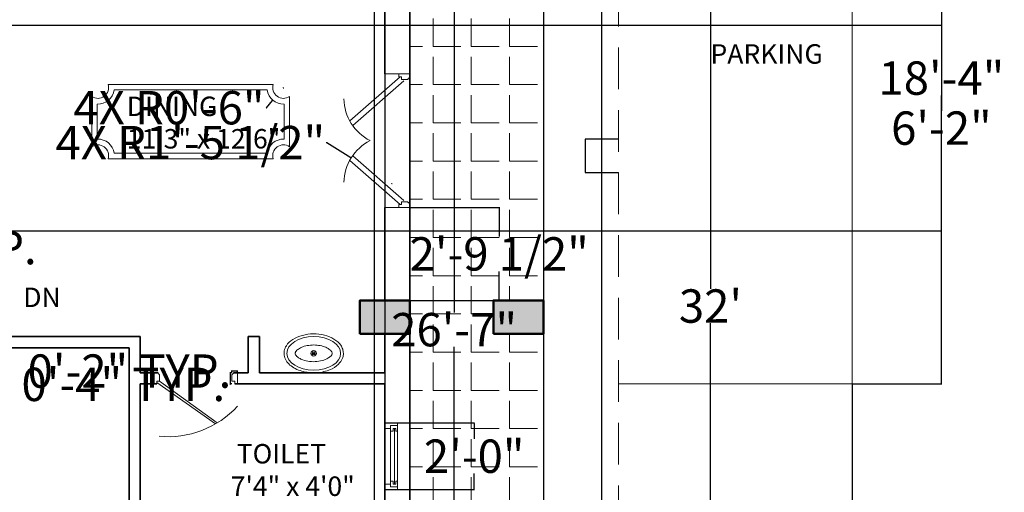
# Model space of a CAD drawing. Units: inches. Extents: x 1063 to 2718, y 423 to 1923.
# Tile 3 of 7: x 1268 to 1622, y 692 to 862. Entities that reach past the tile are written whole.
import ezdxf

# ---------------------------------------------------------------- set-up
doc = ezdxf.new("R2010")
doc.units = ezdxf.units.IN
doc.header["$LTSCALE"] = 6
doc.header["$MEASUREMENT"] = 0
doc.linetypes.add('HIDDEN', pattern=[0.375, 0.25, -0.125])
for name, color, linetype, lineweight in [('A-ANNO-DIMS', 2, 'Continuous', 18), ('A-ANNO-TEXT', 7, 'Continuous', 18), ('A-AREA-IDEN', 7, 'Continuous', 18), ('A-COLS', 7, 'Continuous', 50), ('A-COLS-PATT', 252, 'Continuous', 13), ('A-DOOR', 2, 'Continuous', 18), ('A-FLOR', 7, 'Continuous', 25), ('A-FLOR-FIXT', 4, 'Continuous', 18), ('A-FLOR-PATT', 9, 'Continuous', 13), ('A-FURN', 4, 'Continuous', 18), ('A-GLAZ', 4, 'Continuous', 18), ('A-WALL', 7, 'Continuous', 35), ('C-PKNG', 7, 'Continuous', 18), ('C-PROP', 7, 'Continuous', 25), ('C-PROP-HIDN', 7, 'HIDDEN', 18)]:
    doc.layers.add(name, color=color, linetype=linetype, lineweight=lineweight)
doc.styles.get("Standard").update_dxf_attribs({"font": 'arial.ttf'})
doc.dimstyles.get("Standard").update_dxf_attribs({"dimtxt": 12, "dimasz": 0.18, "dimexe": 0.18, "dimexo": 0.0625, "dimgap": 0.09, "dimtad": 0, "dimtih": 1, "dimtoh": 1, "dimdec": 1, "dimzin": 0, "dimdsep": 46, "dimlunit": 3, "dimtxsty": 'Standard', "dimcen": 0.09, "dimadec": 0, "dimazin": 0, "dimtfac": 1, "dimtdec": 1, "dimtofl": 0, "dimtmove": 0, "dimatfit": 3, "dimfxl": 1, "dimtolj": 1, "dimtzin": 0, "dimarcsym": 0})

# ---------------------------------------------------------------- blocks, each defined once
blk = doc.blocks.new('*D3')
at = {"layer": 'A-ANNO-DIMS', "color": 0, "lineweight": -2, "ltscale": 6, "transparency": 16777216}
for p, q in [((1482.99, 951.12), (1516.18, 951.12)), ((1516, 950.94), (1516, 765.34)), ((1516, 567.3), (1516, 752.9)), ((1482.99, 567.12), (1516.18, 567.12))]:
    blk.add_line(p, q, dxfattribs=at)
at = {"layer": 'A-ANNO-DIMS', "color": 0, "ltscale": 6, "transparency": 16777216}
for points in [[(1515.97, 950.94), (1516.03, 950.94), (1516, 951.12)], [(1515.97, 567.3), (1516.03, 567.3), (1516, 567.12)]]:
    blk.add_solid(points, dxfattribs=at)
at = {"layer": 'Defpoints', "color": 0, "ltscale": 6, "transparency": 16777216}
for p in [(1482.93, 951.12), (1516, 951.12), (1482.93, 567.12)]:
    blk.add_point(p, dxfattribs=at)
at = {"layer": 'A-ANNO-DIMS', "color": 0, "ltscale": 6, "transparency": 16777216, "insert": (1516, 759.12), "char_height": 12, "attachment_point": 5}
blk.add_mtext("\\A1;32'", dxfattribs=at)
blk = doc.blocks.new('DOOR-48-DOUBLE-SWING')
at = {"ltscale": 6}
for p, q in [((20.22, 47), (2.07, 31.16)), ((19.72, 48), (19.72, 47)), ((19.72, 47), (20.72, 47)), ((20.72, 47), (20.72, 46)), ((23.19, 46.24), (23.03, 46.24)), ((23.03, 46.24), (23.03, 46)), ((23.72, 46.54), (23.39, 46.54)), ((23.39, 46.54), (23.39, 46.44)), ((21.53, 45.49), (3.14, 29.43)), ((20.72, 46), (23.03, 46)), ((21.53, 2.51), (3.14, 18.57)), ((20.22, 1), (2.07, 16.84)), ((19.72, 0), (19.72, 1)), ((19.72, 1), (20.72, 1)), ((20.72, 1), (20.72, 2)), ((20.72, 2), (23.03, 2)), ((23.03, 1.76), (23.03, 2)), ((23.19, 1.76), (23.03, 1.76)), ((23.39, 1.46), (23.39, 1.56)), ((23.72, 1.46), (23.39, 1.46))]:
    blk.add_line(p, q, dxfattribs=at)
for p, q in [((14.72, 48), (23.72, 48)), ((23.72, 0), (14.72, 0))]:
    blk.add_line(p, q)
for centre, radius, start, end in [((23.19, 46.44), 0.2, 270, 0), ((17.26, 39.37), 17.27, 181.2158, 242.8966), ((17.26, 8.63), 17.27, 117.1034, 178.7842), ((23.19, 1.56), 0.2, 0, 90)]:
    blk.add_arc(centre, radius, start, end, dxfattribs=at)
blk = doc.blocks.new('DOOR-JAMB-4')
at = {"ltscale": 6}
for p, q in [((0, 0), (0, 4)), ((1, 4), (1, 3)), ((1, 3), (2, 3)), ((1.46, 0), (1.46, 0.33)), ((1.46, 0.33), (1.56, 0.33)), ((1.76, 0.53), (1.76, 0.69)), ((1.76, 0.69), (2, 0.69)), ((2, 3), (2, 0.69))]:
    blk.add_line(p, q, dxfattribs=at)
blk.add_arc((1.56, 0.53), 0.2, 270, 0, dxfattribs=at)
blk = doc.blocks.new('COLUMN-18X12')
blk.add_lwpolyline([(0, 0), (18, 0), (18, 12), (0, 12)], close=True)
blk = doc.blocks.new('PIER-12X12-INLINE')
blk.add_lwpolyline([(0, 0), (12, 0), (12, 12), (0, 12)])
blk = doc.blocks.new('*D28')
at = {"layer": 'A-ANNO-DIMS', "color": 0, "lineweight": -2, "ltscale": 6, "transparency": 16777216}
for p, q in [((1174.86, 804.12), (1167.55, 804.12)), ((1167.73, 803.94), (1167.73, 786.42)), ((1167.73, 756.3), (1167.73, 773.82)), ((1174.86, 756.12), (1167.55, 756.12))]:
    blk.add_line(p, q, dxfattribs=at)
at = {"layer": 'A-ANNO-DIMS', "color": 0, "ltscale": 6, "transparency": 16777216}
for points in [[(1167.7, 803.94), (1167.76, 803.94), (1167.73, 804.12)], [(1167.7, 756.3), (1167.76, 756.3), (1167.73, 756.12)]]:
    blk.add_solid(points, dxfattribs=at)
at = {"layer": 'Defpoints', "color": 0, "ltscale": 6, "transparency": 16777216}
for p in [(1174.93, 804.12), (1167.73, 756.12), (1174.93, 756.12)]:
    blk.add_point(p, dxfattribs=at)
at = {"layer": 'A-ANNO-DIMS', "color": 0, "ltscale": 6, "transparency": 16777216, "insert": (1167.73, 780.12), "char_height": 12, "attachment_point": 5}
blk.add_mtext('\\A1;SLIDING WINDOW 4\'-0" TYP.', dxfattribs=at)
blk = doc.blocks.new('*D32')
at = {"layer": 'A-ANNO-DIMS', "color": 0, "lineweight": -2, "ltscale": 6, "transparency": 16777216}
for p, q in [((1343.86, 735.12), (1343.15, 735.12)), ((1343.33, 734.94), (1343.33, 731.3)), ((1343.86, 731.12), (1343.15, 731.12)), ((1343.33, 730.94), (1343.15, 730.94)), ((1343.33, 731.12), (1343.33, 730.94))]:
    blk.add_line(p, q, dxfattribs=at)
at = {"layer": 'A-ANNO-DIMS', "color": 0, "ltscale": 6, "transparency": 16777216}
for points in [[(1343.3, 734.94), (1343.36, 734.94), (1343.33, 735.12)], [(1343.3, 731.3), (1343.36, 731.3), (1343.33, 731.12)]]:
    blk.add_solid(points, dxfattribs=at)
at = {"layer": 'Defpoints', "color": 0, "ltscale": 6, "transparency": 16777216}
for p in [(1343.93, 735.12), (1343.33, 731.12), (1343.93, 731.12)]:
    blk.add_point(p, dxfattribs=at)
at = {"layer": 'A-ANNO-DIMS', "color": 0, "ltscale": 6, "transparency": 16777216, "insert": (1281.68, 730.94), "char_height": 12, "attachment_point": 5}
blk.add_mtext('\\A1;JAMB 0\'-4" TYP.', dxfattribs=at)
blk = doc.blocks.new('*D33')
at = {"layer": 'A-ANNO-DIMS', "color": 0, "lineweight": -2, "ltscale": 6, "transparency": 16777216}
for p, q in [((1343.93, 735.72), (1343.75, 735.72)), ((1343.93, 735.18), (1343.93, 735.9)), ((1345.75, 735.72), (1344.11, 735.72)), ((1345.93, 735.18), (1345.93, 735.9))]:
    blk.add_line(p, q, dxfattribs=at)
at = {"layer": 'A-ANNO-DIMS', "color": 0, "ltscale": 6, "transparency": 16777216}
for points in [[(1344.11, 735.75), (1344.11, 735.69), (1343.93, 735.72)], [(1345.75, 735.75), (1345.75, 735.69), (1345.93, 735.72)]]:
    blk.add_solid(points, dxfattribs=at)
at = {"layer": 'Defpoints', "color": 0, "ltscale": 6, "transparency": 16777216}
for p in [(1343.93, 735.72), (1343.93, 735.12), (1345.93, 735.12)]:
    blk.add_point(p, dxfattribs=at)
at = {"layer": 'A-ANNO-DIMS', "color": 0, "ltscale": 6, "transparency": 16777216, "insert": (1307.08, 735.72), "char_height": 12, "attachment_point": 5}
blk.add_mtext('\\A1;0\'-2" TYP.', dxfattribs=at)
blk = doc.blocks.new('*D42')
at = {"layer": 'A-ANNO-DIMS', "color": 0, "lineweight": -2, "ltscale": 6, "transparency": 16777216}
for p, q in [((1265.93, 901.06), (1265.93, 895.69)), ((1300.93, 901.06), (1300.93, 895.69)), ((1266.11, 895.87), (1300.75, 895.87)), ((1300.93, 895.87), (1301.11, 895.87))]:
    blk.add_line(p, q, dxfattribs=at)
at = {"layer": 'A-ANNO-DIMS', "color": 0, "ltscale": 6, "transparency": 16777216}
for points in [[(1266.11, 895.9), (1266.11, 895.84), (1265.93, 895.87)], [(1300.75, 895.9), (1300.75, 895.84), (1300.93, 895.87)]]:
    blk.add_solid(points, dxfattribs=at)
at = {"layer": 'Defpoints', "color": 0, "ltscale": 6, "transparency": 16777216}
for p in [(1265.93, 901.12), (1300.93, 901.12), (1300.93, 895.87)]:
    blk.add_point(p, dxfattribs=at)
at = {"layer": 'A-ANNO-DIMS', "color": 0, "ltscale": 6, "transparency": 16777216, "insert": (1398.77, 895.87), "char_height": 12, "attachment_point": 5}
blk.add_mtext('\\A1;SINGLE LEAF 2\'-11" TYP.', dxfattribs=at)
blk = doc.blocks.new('*D49')
at = {"layer": 'A-ANNO-DIMS', "color": 0, "lineweight": -2, "ltscale": 6, "transparency": 16777216}
for p, q in [((1566.99, 951.12), (1599.21, 951.12)), ((1599.03, 950.94), (1599.03, 847.34)), ((1599.03, 731.3), (1599.03, 834.9)), ((1566.99, 731.12), (1599.21, 731.12))]:
    blk.add_line(p, q, dxfattribs=at)
at = {"layer": 'A-ANNO-DIMS', "color": 0, "ltscale": 6, "transparency": 16777216}
for points in [[(1599, 950.94), (1599.06, 950.94), (1599.03, 951.12)], [(1599, 731.3), (1599.06, 731.3), (1599.03, 731.12)]]:
    blk.add_solid(points, dxfattribs=at)
at = {"layer": 'Defpoints', "color": 0, "ltscale": 6, "transparency": 16777216}
for p in [(1566.93, 951.12), (1599.03, 951.12), (1566.93, 731.12)]:
    blk.add_point(p, dxfattribs=at)
at = {"layer": 'A-ANNO-DIMS', "color": 0, "ltscale": 6, "transparency": 16777216, "insert": (1599.03, 841.12), "char_height": 12, "attachment_point": 5}
blk.add_mtext('\\A1;18\'-4"', dxfattribs=at)
blk = doc.blocks.new('*D50')
at = {"layer": 'A-ANNO-DIMS', "color": 0, "lineweight": -2, "ltscale": 6, "transparency": 16777216}
for p, q in [((1566.93, 731.06), (1566.93, 431.18)), ((1150.93, 567.06), (1150.93, 431.18)), ((1151.11, 431.36), (1338.23, 431.36)), ((1566.75, 431.36), (1379.62, 431.36))]:
    blk.add_line(p, q, dxfattribs=at)
at = {"layer": 'A-ANNO-DIMS', "color": 0, "ltscale": 6, "transparency": 16777216}
for points in [[(1151.11, 431.39), (1151.11, 431.33), (1150.93, 431.36)], [(1566.75, 431.39), (1566.75, 431.33), (1566.93, 431.36)]]:
    blk.add_solid(points, dxfattribs=at)
at = {"layer": 'Defpoints', "color": 0, "ltscale": 6, "transparency": 16777216}
for p in [(1566.93, 731.12), (1150.93, 567.12), (1566.93, 431.36)]:
    blk.add_point(p, dxfattribs=at)
at = {"layer": 'A-ANNO-DIMS', "color": 0, "ltscale": 6, "transparency": 16777216, "insert": (1358.93, 431.36), "char_height": 12, "attachment_point": 5}
blk.add_mtext('\\A1;34\'-8"', dxfattribs=at)
blk = doc.blocks.new('*D52')
at = {"layer": 'A-ANNO-DIMS', "color": 0, "lineweight": -2, "ltscale": 6, "transparency": 16777216}
for p, q in [((1455.86, 910.12), (1423.65, 910.12)), ((1423.83, 909.94), (1423.83, 756.84)), ((1423.83, 591.3), (1423.83, 744.4)), ((1455.86, 591.12), (1423.65, 591.12))]:
    blk.add_line(p, q, dxfattribs=at)
at = {"layer": 'A-ANNO-DIMS', "color": 0, "ltscale": 6, "transparency": 16777216}
for points in [[(1423.8, 909.94), (1423.86, 909.94), (1423.83, 910.12)], [(1423.8, 591.3), (1423.86, 591.3), (1423.83, 591.12)]]:
    blk.add_solid(points, dxfattribs=at)
at = {"layer": 'Defpoints', "color": 0, "ltscale": 6, "transparency": 16777216}
for p in [(1423.83, 910.12), (1455.93, 910.12), (1455.93, 591.12)]:
    blk.add_point(p, dxfattribs=at)
at = {"layer": 'A-ANNO-DIMS', "color": 0, "ltscale": 6, "transparency": 16777216, "insert": (1423.83, 750.62), "char_height": 12, "attachment_point": 5}
blk.add_mtext('\\A1;26\'-7"', dxfattribs=at)
blk = doc.blocks.new('*D54')
at = {"layer": 'A-ANNO-DIMS', "color": 0, "lineweight": -2, "ltscale": 6, "transparency": 16777216}
for p, q in [((1227.99, 860.12), (1599.21, 860.12)), ((1599.03, 859.94), (1599.03, 829.34)), ((1599.03, 786.3), (1599.03, 816.9)), ((1227.99, 786.12), (1599.21, 786.12))]:
    blk.add_line(p, q, dxfattribs=at)
at = {"layer": 'A-ANNO-DIMS', "color": 0, "ltscale": 6, "transparency": 16777216}
for points in [[(1599, 859.94), (1599.06, 859.94), (1599.03, 860.12)], [(1599, 786.3), (1599.06, 786.3), (1599.03, 786.12)]]:
    blk.add_solid(points, dxfattribs=at)
at = {"layer": 'Defpoints', "color": 0, "ltscale": 6, "transparency": 16777216}
for p in [(1227.93, 860.12), (1227.93, 786.12), (1599.03, 786.12)]:
    blk.add_point(p, dxfattribs=at)
at = {"layer": 'A-ANNO-DIMS', "color": 0, "ltscale": 6, "transparency": 16777216, "insert": (1599.03, 823.12), "char_height": 12, "attachment_point": 5}
blk.add_mtext('\\A1;6\'-2"', dxfattribs=at)
blk = doc.blocks.new('*D65')
at = {"layer": 'A-ANNO-DIMS', "color": 0, "lineweight": -2, "ltscale": 6, "transparency": 16777216}
for p, q in [((1395.08, 961.04), (1395.08, 431.18)), ((1398.93, 954.06), (1398.93, 431.18)), ((1395.26, 431.36), (1398.75, 431.36)), ((1398.93, 431.36), (1399.11, 431.36))]:
    blk.add_line(p, q, dxfattribs=at)
at = {"layer": 'A-ANNO-DIMS', "color": 0, "ltscale": 6, "transparency": 16777216}
for points in [[(1395.26, 431.39), (1395.26, 431.33), (1395.08, 431.36)], [(1398.75, 431.39), (1398.75, 431.33), (1398.93, 431.36)]]:
    blk.add_solid(points, dxfattribs=at)
at = {"layer": 'Defpoints', "color": 0, "ltscale": 6, "transparency": 16777216}
for p in [(1395.08, 961.11), (1398.93, 954.12), (1398.93, 431.36)]:
    blk.add_point(p, dxfattribs=at)
at = {"layer": 'A-ANNO-DIMS', "color": 0, "ltscale": 6, "transparency": 16777216, "insert": (1415.15, 431.36), "char_height": 12, "attachment_point": 5}
blk.add_mtext('\\A1;0\'-4"', dxfattribs=at)
blk = doc.blocks.new('*D70')
at = {"layer": 'A-ANNO-DIMS', "color": 0, "lineweight": -2, "ltscale": 6, "transparency": 16777216}
for p, q in [((1398.99, 717.1), (1431.21, 717.1)), ((1431.03, 716.92), (1431.03, 711.32)), ((1431.03, 693.28), (1431.03, 698.88)), ((1398.99, 693.1), (1431.21, 693.1))]:
    blk.add_line(p, q, dxfattribs=at)
at = {"layer": 'A-ANNO-DIMS', "color": 0, "ltscale": 6, "transparency": 16777216}
for points in [[(1431, 716.92), (1431.06, 716.92), (1431.03, 717.1)], [(1431, 693.28), (1431.06, 693.28), (1431.03, 693.1)]]:
    blk.add_solid(points, dxfattribs=at)
at = {"layer": 'Defpoints', "color": 0, "ltscale": 6, "transparency": 16777216}
for p in [(1398.93, 717.1), (1398.93, 693.1), (1431.03, 693.1)]:
    blk.add_point(p, dxfattribs=at)
at = {"layer": 'A-ANNO-DIMS', "color": 0, "ltscale": 6, "transparency": 16777216, "insert": (1431.03, 705.1), "char_height": 12, "attachment_point": 5}
blk.add_mtext('\\A1;2\'-0"', dxfattribs=at)
blk = doc.blocks.new('*D71')
at = {"layer": 'A-ANNO-DIMS', "color": 0, "lineweight": -2, "ltscale": 6, "transparency": 16777216}
for p, q in [((1407.99, 794.62), (1440.21, 794.62)), ((1440.03, 794.44), (1440.03, 784.16)), ((1440.03, 761.29), (1440.03, 771.57)), ((1407.99, 761.11), (1440.21, 761.11))]:
    blk.add_line(p, q, dxfattribs=at)
at = {"layer": 'A-ANNO-DIMS', "color": 0, "ltscale": 6, "transparency": 16777216}
for points in [[(1440, 794.44), (1440.06, 794.44), (1440.03, 794.62)], [(1440, 761.29), (1440.06, 761.29), (1440.03, 761.11)]]:
    blk.add_solid(points, dxfattribs=at)
at = {"layer": 'Defpoints', "color": 0, "ltscale": 6, "transparency": 16777216}
for p in [(1407.93, 794.62), (1407.93, 761.11), (1440.03, 761.11)]:
    blk.add_point(p, dxfattribs=at)
at = {"layer": 'A-ANNO-DIMS', "color": 0, "ltscale": 6, "transparency": 16777216, "insert": (1440.03, 777.87), "char_height": 12, "attachment_point": 5}
blk.add_mtext('\\A1;2\'-9 1/2"', dxfattribs=at)
blk = doc.blocks.new('*D74')
at = {"layer": 'A-ANNO-DIMS', "color": 0, "lineweight": -2, "ltscale": 6, "transparency": 16777216}
for p, q in [((1377.88, 817.91), (1378.06, 817.91)), ((1378.06, 817.91), (1386.68, 812.51)), ((1401.38, 803.25), (1401.56, 803.25)), ((1401.47, 803.16), (1401.47, 803.34))]:
    blk.add_line(p, q, dxfattribs=at)
at = {"layer": 'A-ANNO-DIMS', "color": 0, "ltscale": 6, "transparency": 16777216}
blk.add_solid([(1386.7, 812.53), (1386.67, 812.48), (1386.84, 812.41)], dxfattribs=at)
at = {"layer": 'Defpoints', "color": 0, "ltscale": 6, "transparency": 16777216}
for p in [(1386.84, 812.41), (1401.47, 803.25)]:
    blk.add_point(p, dxfattribs=at)
at = {"layer": 'A-ANNO-DIMS', "color": 0, "ltscale": 6, "transparency": 16777216, "insert": (1328.98, 817.91), "char_height": 12, "attachment_point": 5}
blk.add_mtext('\\A1;4X R1\'-5 1/2"', dxfattribs=at)
blk = doc.blocks.new('*D75')
at = {"layer": 'A-ANNO-DIMS', "color": 0, "lineweight": -2, "ltscale": 6, "transparency": 16777216}
for p, q in [((1362.37, 837.65), (1362.55, 837.65)), ((1362.46, 837.56), (1362.46, 837.74)), ((1356.4, 830.45), (1358.56, 833.01)), ((1356.22, 830.45), (1356.4, 830.45))]:
    blk.add_line(p, q, dxfattribs=at)
at = {"layer": 'A-ANNO-DIMS', "color": 0, "ltscale": 6, "transparency": 16777216}
blk.add_solid([(1358.54, 833.03), (1358.58, 832.99), (1358.67, 833.15)], dxfattribs=at)
at = {"layer": 'Defpoints', "color": 0, "ltscale": 6, "transparency": 16777216}
for p in [(1362.46, 837.65), (1358.67, 833.15)]:
    blk.add_point(p, dxfattribs=at)
at = {"layer": 'A-ANNO-DIMS', "color": 0, "ltscale": 6, "transparency": 16777216, "insert": (1321.3, 830.45), "char_height": 12, "attachment_point": 5}
blk.add_mtext('\\A1;4X R0\'-6"', dxfattribs=at)

msp = doc.modelspace()

# ---------------------------------------------------------------- hatches: boundary and pattern name
at = {"layer": 'A-COLS-PATT', "ltscale": 6}
h = msp.add_hatch(color=256, dxfattribs=at)
h.dxf.hatch_style = 1
h.paths.add_polyline_path([(1192.93, 603.12), (1174.93, 603.12), (1174.93, 591.12), (1192.93, 591.12)])
h.paths.add_polyline_path([(1407.93, 603.12), (1389.93, 603.12), (1389.93, 591.12), (1407.93, 591.12)])
h.paths.add_polyline_path([(1192.93, 756.12), (1174.93, 756.12), (1174.93, 744.12), (1192.93, 744.12)])
h.paths.add_polyline_path([(1407.93, 761.11), (1389.93, 761.11), (1389.93, 749.11), (1407.93, 749.11)])
h.paths.add_polyline_path([(1455.93, 761.11), (1437.93, 761.11), (1437.93, 749.11), (1455.93, 749.11)])
h.paths.add_polyline_path([(1455.93, 910.12), (1437.93, 910.12), (1437.93, 898.12), (1455.93, 898.12)])
h.paths.add_polyline_path([(1407.93, 910.12), (1389.93, 910.12), (1389.93, 898.12), (1407.93, 898.12)])
h.paths.add_polyline_path([(1192.93, 910.12), (1174.93, 910.12), (1174.93, 898.12), (1192.93, 898.12)])
h.paths.add_polyline_path([(1192.93, 1055.12), (1174.93, 1055.12), (1174.93, 1043.12), (1192.93, 1043.12)])
h.paths.add_polyline_path([(1407.93, 1055.12), (1389.93, 1055.12), (1389.93, 1043.12), (1407.93, 1043.12)])
at = {"layer": 'A-FLOR-PATT', "ltscale": 6}
h = msp.add_hatch(dxfattribs=at)
h.set_pattern_fill('ANGLE', color=256, scale=50)
h.set_pattern_definition([(0, (0, 0), (0, 13.75), [10, -3.75]), (90, (0, 0), (-13.75, 8e-16), [10, -3.75])])
h.paths.add_polyline_path([(1455.93, 749.11), (1437.93, 749.11), (1437.93, 761.11), (1455.93, 761.11), (1455.93, 868.12), (1407.93, 868.12), (1407.93, 595.12), (1455.93, 595.12)])
h.paths.add_polyline_path([(1377.93, 674.12), (1315.93, 674.12), (1315.93, 600.12), (1377.93, 600.12)])

# ---------------------------------------------------------------- linework, layer by layer
at = {"layer": 'A-DOOR', "ltscale": 6}
for p, q in [((1316.93, 731.62), (1338.02, 716.72)), ((1317.93, 732.12), (1338.68, 717.11))]:
    msp.add_line(p, q, dxfattribs=at)
msp.add_arc((1320.91, 746.15), 34.04, 264.6951, 317.3946, dxfattribs=at)
at = {"layer": 'A-FLOR'}
msp.add_line((1455.93, 898.12), (1455.93, 591.12), dxfattribs=at)
at = {"layer": 'A-FLOR-FIXT', "ltscale": 6}
for p, q in [((1373.88, 742.1), (1372.8, 742.1)), ((1373.34, 742.64), (1373.34, 741.56))]:
    msp.add_line(p, q, dxfattribs=at)
for radius in [0.987, 0.539]:
    msp.add_circle((1373.34, 742.1), radius, dxfattribs=at)
msp.add_ellipse((1373.34, 742.1), major_axis=(9.67, 0), ratio=0.620608, dxfattribs=at)
for points, knots in [([(1384.01, 742.1), (1384.01, 742.61), (1383.92, 743.12), (1383.61, 744.09), (1383.37, 744.56), (1382.48, 745.87), (1381.64, 746.62), (1379.63, 747.85), (1378.45, 748.32), (1375.92, 748.96), (1374.56, 749.11), (1371.86, 749.09), (1370.51, 748.91), (1368, 748.24), (1366.84, 747.75), (1364.87, 746.49), (1364.06, 745.72), (1363.13, 744.25), (1362.87, 743.61), (1362.63, 742.29), (1362.65, 741.61), (1362.97, 740.3), (1363.27, 739.68), (1364.09, 738.53), (1364.6, 738.01), (1366.41, 736.62), (1367.96, 735.93), (1371.37, 735.12), (1373.22, 735), (1376.8, 735.37), (1378.51, 735.85), (1381.08, 737.16), (1382.04, 737.9), (1383.22, 739.35), (1383.57, 739.99), (1383.93, 741.13), (1384.01, 741.61), (1384.01, 742.1)], [0, 0, 0, 0, 0.199891, 0.199891, 0.399781, 0.399781, 0.794265, 0.794265, 1.188748, 1.188748, 1.583232, 1.583232, 1.977715, 1.977715, 2.372199, 2.372199, 2.766682, 2.766682, 3.030116, 3.030116, 3.293549, 3.293549, 3.556982, 3.556982, 3.820416, 3.820416, 4.347819, 4.347819, 4.875222, 4.875222, 5.402625, 5.402625, 5.816568, 5.816568, 6.091003, 6.091003, 6.283185, 6.283185, 6.283185, 6.283185]), ([(1380.01, 742.1), (1380.01, 742.17), (1380, 742.25), (1379.94, 742.43), (1379.9, 742.54), (1379.73, 742.81), (1379.61, 742.96), (1379.28, 743.3), (1379.08, 743.47), (1378.4, 743.94), (1377.86, 744.22), (1376.59, 744.68), (1375.87, 744.87), (1374.35, 745.09), (1373.55, 745.13), (1371.97, 745.05), (1371.2, 744.94), (1369.77, 744.59), (1369.13, 744.35), (1368.05, 743.81), (1367.63, 743.51), (1367.1, 743.01), (1366.95, 742.81), (1366.75, 742.48), (1366.71, 742.35), (1366.67, 742.15), (1366.67, 742.07), (1366.7, 741.87), (1366.74, 741.75), (1366.92, 741.43), (1367.07, 741.23), (1367.51, 740.81), (1367.8, 740.58), (1368.52, 740.15), (1368.94, 739.94), (1370.14, 739.5), (1370.97, 739.3), (1372.71, 739.09), (1373.63, 739.07), (1375.39, 739.24), (1376.24, 739.42), (1377.73, 739.92), (1378.36, 740.24), (1379.18, 740.8), (1379.44, 741.04), (1379.79, 741.47), (1379.89, 741.65), (1379.99, 741.92), (1380.01, 742.01), (1380.01, 742.1)], [0, 0, 0, 0, 0.18324, 0.18324, 0.366481, 0.366481, 0.549721, 0.549721, 0.732962, 0.732962, 1.037063, 1.037063, 1.341164, 1.341164, 1.645265, 1.645265, 1.949367, 1.949367, 2.253468, 2.253468, 2.557569, 2.557569, 2.788449, 2.788449, 3.019329, 3.019329, 3.250209, 3.250209, 3.481089, 3.481089, 3.711969, 3.711969, 3.942849, 3.942849, 4.173729, 4.173729, 4.518554, 4.518554, 4.863378, 4.863378, 5.208203, 5.208203, 5.553027, 5.553027, 5.802313, 5.802313, 6.051598, 6.051598, 6.283185, 6.283185, 6.283185, 6.283185])]:
    msp.add_open_spline(points, degree=3, knots=knots, dxfattribs=at)
at = {"layer": 'A-FURN', "ltscale": 6}
for p, q in [((1299.39, 838.86), (1358.82, 838.86)), ((1301.58, 836.86), (1356.63, 836.86)), ((1293.53, 816.41), (1293.53, 834.52)), ((1364.68, 834.52), (1364.68, 816.41)), ((1295.53, 819.15), (1295.53, 831.77)), ((1362.68, 831.77), (1362.68, 819.15)), ((1358.82, 812.06), (1299.39, 812.06)), ((1356.63, 814.06), (1301.58, 814.06))]:
    msp.add_line(p, q, dxfattribs=at)
for centre, radius, start, end in [((1295.74, 837.65), 3.84, 234.8003, 18.3164), ((1295.74, 837.65), 5.89, 267.9212, 352.2551), ((1362.46, 837.65), 5.89, 187.7449, 272.0788), ((1362.46, 837.65), 3.84, 161.6836, 305.1997), ((1295.74, 813.27), 5.89, 7.7449, 92.0788), ((1362.46, 813.27), 5.89, 87.9212, 172.2551), ((1295.74, 813.27), 3.84, 341.6836, 125.1997), ((1362.46, 813.27), 3.84, 54.8003, 198.3164)]:
    msp.add_arc(centre, radius, start, end, dxfattribs=at)
at = {"layer": 'A-GLAZ', "ltscale": 6}
for p, q in [((1398.93, 717.1), (1398.93, 715.1)), ((1400.93, 715.1), (1400.93, 716.1)), ((1400.93, 716.1), (1403.43, 716.1)), ((1403.43, 717.1), (1403.43, 693.1)), ((1403.43, 694.1), (1403.43, 716.1)), ((1398.93, 715.1), (1400.93, 715.1)), ((1400.93, 695.1), (1400.93, 715.1)), ((1400.93, 715.1), (1400.93, 714.1)), ((1400.93, 714.1), (1401.93, 714.1)), ((1401.93, 714.1), (1401.93, 715.1)), ((1401.93, 715.1), (1402.93, 715.1)), ((1402.43, 695.1), (1402.43, 715.1)), ((1402.93, 715.1), (1402.93, 714.1)), ((1402.93, 714.1), (1403.43, 714.1)), ((1398.93, 693.1), (1398.93, 695.1)), ((1398.93, 695.1), (1400.93, 695.1)), ((1400.93, 695.1), (1400.93, 696.1)), ((1400.93, 696.1), (1401.93, 696.1)), ((1400.93, 695.1), (1400.93, 694.1)), ((1400.93, 694.1), (1403.43, 694.1)), ((1401.93, 696.1), (1401.93, 695.1)), ((1401.93, 695.1), (1402.93, 695.1)), ((1402.93, 695.1), (1402.93, 696.1)), ((1402.93, 696.1), (1403.43, 696.1))]:
    msp.add_line(p, q, dxfattribs=at)
msp.add_lwpolyline([(1407.93, 693.1), (1407.93, 717.1), (1398.93, 717.1), (1398.93, 693.1)], close=True, dxfattribs=at)
at = {"layer": 'A-WALL', "ltscale": 6}
for p, q in [((1407.93, 1055.12), (1407.93, 591.12)), ((1349.83, 735.12), (1349.83, 748.12)), ((1349.83, 748.12), (1353.83, 748.12)), ((1353.83, 735.12), (1353.83, 748.12)), ((1398.93, 731.12), (1344.93, 731.12))]:
    msp.add_line(p, q, dxfattribs=at)
at = {"layer": 'A-WALL'}
for p, q in [((1398.93, 898.12), (1398.93, 842.62)), ((1398.93, 794.62), (1398.93, 761.11)), ((1310.93, 748.12), (1192.93, 748.12)), ((1310.93, 748.12), (1310.93, 735.12)), ((1398.93, 749.11), (1398.93, 735.12)), ((1306.93, 744.12), (1183.93, 744.12)), ((1306.93, 744.12), (1306.93, 655.12)), ((1310.93, 735.12), (1317.39, 735.12)), ((1344.46, 735.12), (1349.83, 735.12)), ((1353.83, 735.12), (1398.93, 735.12)), ((1310.93, 731.12), (1316.93, 731.12)), ((1310.93, 731.12), (1310.93, 683.12)), ((1398.93, 731.12), (1398.93, 683.12))]:
    msp.add_line(p, q, dxfattribs=at)
at = {"layer": 'C-PKNG', "ltscale": 6}
for p, q in [((1566.93, 731.12), (1566.93, 951.12)), ((1482.93, 731.12), (1566.93, 731.12))]:
    msp.add_line(p, q, dxfattribs=at)
at = {"layer": 'C-PROP'}
msp.add_line((1476.93, 567.12), (1476.93, 945.12), dxfattribs=at)
at = {"layer": 'C-PROP-HIDN', "ltscale": 10}
msp.add_line((1482.93, 567.12), (1482.93, 951.12), dxfattribs=at)

# ---------------------------------------------------------------- block references
at = {"layer": 'A-COLS'}
for p in [(1389.93, 749.11), (1437.93, 749.11)]:
    msp.add_blockref('COLUMN-18X12', p, dxfattribs=at)
at = {"layer": 'A-DOOR'}
msp.add_blockref('DOOR-48-DOUBLE-SWING', (1384.21, 794.62), dxfattribs=at)
at = {"layer": 'A-DOOR', "extrusion": (0, 0, -1), "zscale": -1, "rotation": 180}
msp.add_blockref('DOOR-JAMB-4', (-1315.93, 735.12), dxfattribs=at)
at = {"layer": 'A-DOOR', "rotation": 180}
msp.add_blockref('DOOR-JAMB-4', (1345.93, 735.12), dxfattribs=at)
at = {"layer": 'C-PROP', "rotation": 180}
msp.add_blockref('PIER-12X12-INLINE', (1482.93, 819.12), dxfattribs=at)

# ---------------------------------------------------------------- texts
at = {"layer": 'A-ANNO-TEXT', "ltscale": 6, "insert": (1268.91, 765.75), "char_height": 7, "attachment_point": 1}
msp.add_mtext_dynamic_manual_height_columns('DN', width=175.2385, gutter_width=1, heights=[0], dxfattribs=at)
at = {"layer": 'A-AREA-IDEN', "ltscale": 6, "char_height": 7, "attachment_point": 1}
for s, insert in [('PARKING', (1516, 853.29)), ('DINING\\P11\'3" x 12\'6"', (1306.14, 834.45)), (' TOILET\\P7\'4" x 4\'0"', (1343.51, 709.48))]:
    msp.add_mtext_dynamic_manual_height_columns(s, width=175.2385, gutter_width=1, heights=[0], dxfattribs=dict(at, insert=insert))

# ---------------------------------------------------------------- dimensions: what is measured, and where the dimension line sits
at = {"layer": 'A-ANNO-DIMS', "ltscale": 6}
for base, p1, p2, picture, middle in [((1398.9256, 431.3553), (1395.0779, 961.1073), (1398.9256, 954.1189), '*D65', (1415.1451, 431.3553)), ((1566.93, 431.36), (1150.93, 567.12), (1566.93, 731.12), '*D50', (1358.93, 431.36))]:
    dim = msp.add_linear_dim(base=base, p1=p1, p2=p2, dimstyle='Standard', override={"dimdec": 1, "dimlfac": 1, "dimrnd": 0, "dimzin": 1, "dimdsep": 46, "dimlunit": 4, "dimfrac": 2}, dxfattribs=at)
    dim.commit()
    dim.dimension.update_dxf_attribs({"geometry": picture, "text_midpoint": middle})
for base, p1, p2, angle, override, picture, middle in [((1516, 951.12), (1482.93, 567.12), (1482.93, 951.12), 90, {"dimclrd": 0, "dimclre": 0, "dimclrt": 0}, '*D3', (1516, 759.12)), ((1599.03, 951.12), (1566.93, 731.12), (1566.93, 951.12), 90, {"dimdec": 1, "dimlfac": 1, "dimrnd": 0, "dimzin": 1, "dimdsep": 46, "dimlunit": 4, "dimfrac": 2}, '*D49', (1599.03, 841.12)), ((1423.83, 910.12), (1455.93, 591.12), (1455.93, 910.12), 90, {"dimdec": 1, "dimlfac": 1, "dimrnd": 0, "dimzin": 1, "dimdsep": 46, "dimlunit": 4, "dimfrac": 2}, '*D52', (1423.83, 750.62)), ((1599.03, 786.12), (1227.93, 860.12), (1227.93, 786.12), 90, {"dimdec": 1, "dimlfac": 1, "dimrnd": 0, "dimzin": 1, "dimdsep": 46, "dimlunit": 4, "dimfrac": 2}, '*D54', (1599.03, 823.12)), ((1440.03, 761.11), (1407.93, 794.62), (1407.93, 761.11), 270, {"dimdec": 1, "dimlfac": 1, "dimrnd": 0, "dimzin": 1, "dimdsep": 46, "dimlunit": 4, "dimfrac": 2}, '*D71', (1440.03, 777.87)), ((1431.03, 693.1), (1398.93, 717.1), (1398.93, 693.1), 270, {"dimdec": 1, "dimlfac": 1, "dimrnd": 0, "dimzin": 1, "dimdsep": 46, "dimlunit": 4, "dimfrac": 2}, '*D70', (1431.03, 705.1))]:
    dim = msp.add_linear_dim(base=base, p1=p1, p2=p2, angle=angle, dimstyle='Standard', override=override, dxfattribs=at)
    dim.commit()
    dim.dimension.update_dxf_attribs({"geometry": picture, "text_midpoint": middle})
dim = msp.add_linear_dim(base=(1300.93, 895.87), p1=(1265.93, 901.12), p2=(1300.93, 901.12), text='SINGLE LEAF <> TYP.', dimstyle='Standard', override={"dimdec": 1, "dimlfac": 1, "dimrnd": 0, "dimzin": 1, "dimdsep": 46, "dimlunit": 4, "dimfrac": 2}, dxfattribs=at)
dim.commit()
dim.dimension.update_dxf_attribs({"geometry": '*D42', "text_midpoint": (1398.77, 895.87)})
for center, mpoint, picture, middle in [((1362.46, 837.65), (1358.67, 833.15), '*D75', (1321.3, 830.45)), ((1401.47, 803.25), (1386.84, 812.41), '*D74', (1328.98, 817.91))]:
    dim = msp.add_radius_dim(center=center, mpoint=mpoint, text='4X <>', dimstyle='Standard', override={"dimdec": 1, "dimlfac": 1, "dimrnd": 0, "dimzin": 1, "dimdsep": 46, "dimlunit": 4, "dimfrac": 2}, dxfattribs=at)
    dim.commit()
    dim.dimension.update_dxf_attribs({"geometry": picture, "text_midpoint": middle, "dimtype": 164})
for base, p1, p2, angle, text, picture, middle in [((1167.73, 756.12), (1174.93, 804.12), (1174.93, 756.12), 270, 'SLIDING WINDOW <> TYP.', '*D28', (1167.73, 780.12)), ((1343.33, 731.12), (1343.93, 735.12), (1343.93, 731.12), 270, 'JAMB <> TYP.', '*D32', (1281.68, 730.94)), ((1343.93, 735.72), (1345.93, 735.12), (1343.93, 735.12), 180, '<> TYP.', '*D33', (1307.08, 735.72))]:
    dim = msp.add_linear_dim(base=base, p1=p1, p2=p2, angle=angle, text=text, dimstyle='Standard', override={"dimdec": 1, "dimlfac": 1, "dimrnd": 0, "dimzin": 1, "dimdsep": 46, "dimlunit": 4, "dimfrac": 2}, dxfattribs=at)
    dim.commit()
    dim.dimension.update_dxf_attribs({"geometry": picture, "text_midpoint": middle})

doc.saveas('drawing.dxf')
